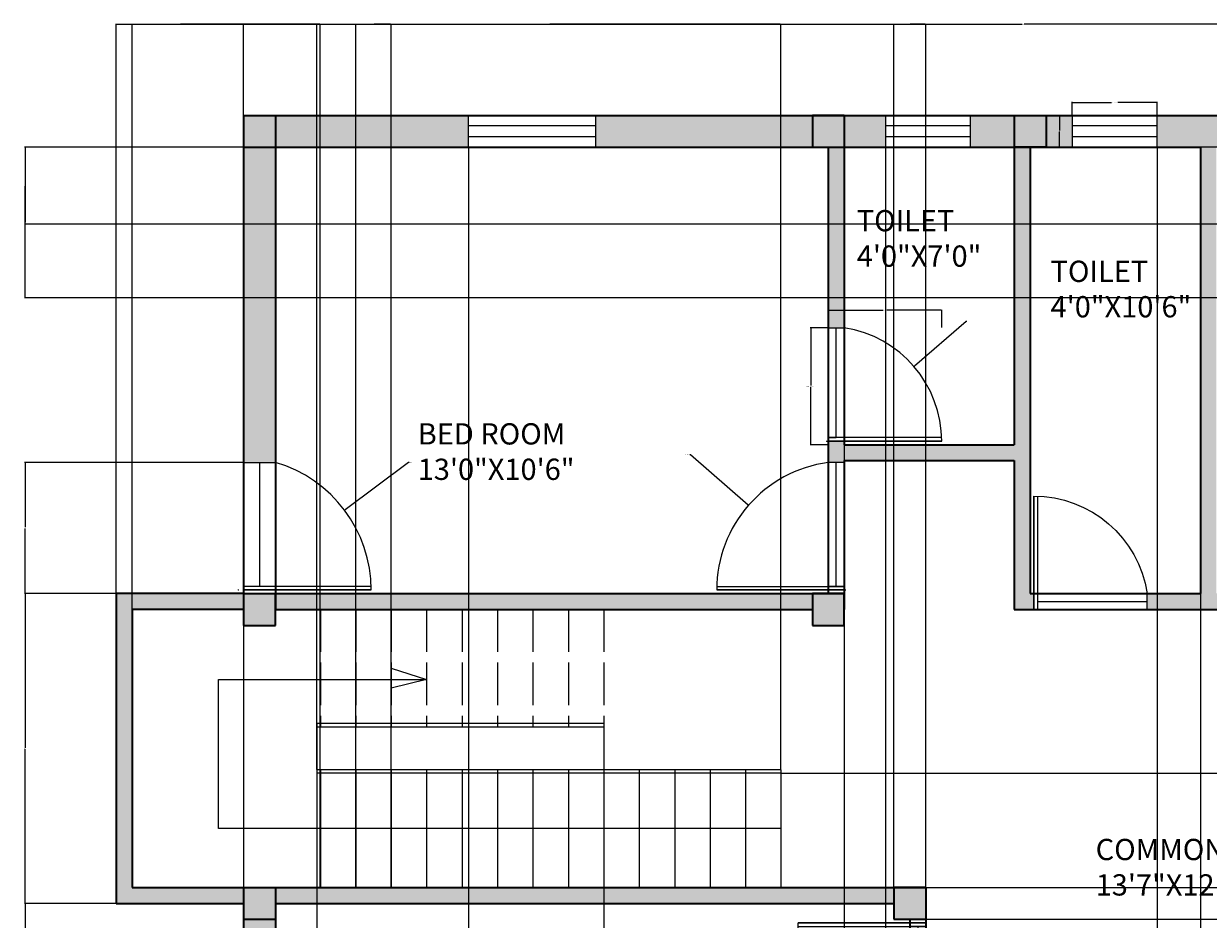
# Model space of a CAD drawing. Units: inches. Extents: x 6217 to 6782, y 16564 to 16973.
# Tile 2 of 3: x 6217 to 6552, y 16720 to 16973. Entities that reach past the tile are written whole.
import ezdxf

# ---------------------------------------------------------------- set-up
doc = ezdxf.new("R2010")
doc.units = ezdxf.units.IN
doc.header["$MEASUREMENT"] = 0
doc.linetypes.add('ACAD_ISO02W100', pattern=[15, 12, -3])
for name, color, linetype, lineweight in [('A-ANNO-DIMS', 2, 'Continuous', 18), ('A-ANNO-SYMB', 7, 'Continuous', 18), ('A-AREA-IDEN', 7, 'Continuous', 18), ('A-COLS', 7, 'Continuous', 35), ('A-DOOR', 3, 'Continuous', 18), ('A-FLOR-STRS', 7, 'Continuous', 25), ('A-FLOR-STRS-OVHD', 7, 'ACAD_ISO02W100', 18), ('A-GLAZ', 4, 'Continuous', 18), ('A-WALL', 7, 'Continuous', 35)]:
    doc.layers.add(name, color=color, linetype=linetype, lineweight=lineweight)
doc.layers.add('A-COLS-PATT', color=252, linetype='Continuous', lineweight=13, true_color=0x939598)
doc.layers.add('A-WALL-PATT', color=146, linetype='Continuous', lineweight=13, true_color=0x105689)
doc.styles.get("Standard").update_dxf_attribs({"font": 'arial.ttf'})
doc.dimstyles.get("Standard").update_dxf_attribs({"dimtxt": 0.18, "dimasz": 0.18, "dimexe": 0.18, "dimexo": 0.0625, "dimgap": 0.09, "dimtad": 0, "dimtih": 1, "dimtoh": 1, "dimdec": 4, "dimzin": 0, "dimdsep": 46, "dimtxsty": 'Standard', "dimcen": 0.09, "dimadec": 0, "dimazin": 0, "dimtfac": 1, "dimtdec": 4, "dimtofl": 0, "dimtmove": 0, "dimatfit": 3, "dimfxl": 1, "dimtolj": 1, "dimtzin": 0, "dimarcsym": 0})

# ---------------------------------------------------------------- blocks, each defined once
blk = doc.blocks.new('WIN-36')
for p, q in [((0, 9), (0, 0)), ((36, 9), (0, 9)), ((36, 0), (36, 9)), ((36, 6), (0, 6)), ((0, 3), (36, 3)), ((0, 0), (36, 0))]:
    blk.add_line(p, q)
blk = doc.blocks.new('VENT-24')
for p, q in [((0, 9), (0, 0)), ((24, 9), (0, 9)), ((24, 0), (24, 9)), ((24, 6), (0, 6)), ((0, 3), (24, 3)), ((0, 0), (24, 0))]:
    blk.add_line(p, q)
blk = doc.blocks.new('DOOR-SINGLE-36-A')
for p, q in [((0, 36), (-4.5, 36)), ((-2.25, 1), (-2.25, 36)), ((0, 0), (0, 36)), ((-36, 1), (0, 1)), ((0, 0), (-36, 0)), ((-36, 0), (0, 0)), ((0, 1), (-4.5, 1)), ((-4.5, 1), (-2.25, 1)), ((0, -1), (0, 0))]:
    blk.add_line(p, q)
blk.add_arc((0.32, 0), 36.32, 97.6281, 180)
blk = doc.blocks.new('DOOR-SINGLE-32')
for p, q in [((0, 0), (0, 32)), ((0, 32), (4.5, 32)), ((2.25, 1), (2.25, 32)), ((32, 1), (0, 1)), ((4.5, 1), (0, 1)), ((0, -1), (0, 0)), ((0, 0), (32, 0)), ((32, 0), (0, 0))]:
    blk.add_line(p, q)
blk.add_arc((-0.37, 0), 32.37, 0, 81.3499)
blk = doc.blocks.new('*D8')
at = {"layer": 'A-ANNO-DIMS', "color": 0, "lineweight": -2, "transparency": 16777216}
for p, q in [((6513.38, 16947.07), (6513.38, 16950.78)), ((6513.56, 16950.6), (6524.48, 16950.6)), ((6537.2, 16950.6), (6526.28, 16950.6)), ((6537.38, 16947.07), (6537.38, 16950.78))]:
    blk.add_line(p, q, dxfattribs=at)
at = {"layer": 'A-ANNO-DIMS', "color": 0, "transparency": 16777216}
for points in [[(6513.56, 16950.63), (6513.56, 16950.57), (6513.38, 16950.6)], [(6537.2, 16950.63), (6537.2, 16950.57), (6537.38, 16950.6)]]:
    blk.add_solid(points, dxfattribs=at)
at = {"layer": 'Defpoints', "color": 0, "transparency": 16777216}
for p in [(6513.38, 16950.6), (6513.38, 16947), (6537.38, 16947)]:
    blk.add_point(p, dxfattribs=at)
at = {"layer": 'A-ANNO-DIMS', "color": 0, "transparency": 16777216, "insert": (6525.38, 16950.6), "char_height": 0.18, "attachment_point": 5}
blk.add_mtext('\\A1;VENT 24 TYP.', dxfattribs=at)
blk = doc.blocks.new('*D9')
at = {"layer": 'A-ANNO-DIMS', "color": 0, "lineweight": -2, "transparency": 16777216}
for p, q in [((6513.32, 16947), (6509.6, 16947)), ((6509.78, 16946.82), (6509.78, 16942.69)), ((6509.78, 16938.18), (6509.78, 16942.32)), ((6513.32, 16938), (6509.6, 16938))]:
    blk.add_line(p, q, dxfattribs=at)
at = {"layer": 'A-ANNO-DIMS', "color": 0, "transparency": 16777216}
for points in [[(6509.75, 16946.82), (6509.81, 16946.82), (6509.78, 16947)], [(6509.75, 16938.18), (6509.81, 16938.18), (6509.78, 16938)]]:
    blk.add_solid(points, dxfattribs=at)
at = {"layer": 'Defpoints', "color": 0, "transparency": 16777216}
for p in [(6513.38, 16947), (6509.78, 16938), (6513.38, 16938)]:
    blk.add_point(p, dxfattribs=at)
at = {"layer": 'A-ANNO-DIMS', "color": 0, "transparency": 16777216, "insert": (6509.78, 16942.5), "char_height": 0.18, "attachment_point": 5}
blk.add_mtext('\\A1;9 TYP.', dxfattribs=at)
blk = doc.blocks.new('*D14')
at = {"layer": 'A-ANNO-DIMS', "color": 0, "lineweight": -2, "transparency": 16777216}
for p, q in [((6444.47, 16887), (6439.4, 16887)), ((6439.58, 16886.82), (6439.58, 16870.69)), ((6439.58, 16854.18), (6439.58, 16870.32)), ((6444.47, 16854), (6439.4, 16854))]:
    blk.add_line(p, q, dxfattribs=at)
at = {"layer": 'A-ANNO-DIMS', "color": 0, "transparency": 16777216}
for points in [[(6439.55, 16886.82), (6439.61, 16886.82), (6439.58, 16887)], [(6439.55, 16854.18), (6439.61, 16854.18), (6439.58, 16854)]]:
    blk.add_solid(points, dxfattribs=at)
at = {"layer": 'Defpoints', "color": 0, "transparency": 16777216}
for p in [(6439.58, 16887), (6444.53, 16887), (6444.53, 16854)]:
    blk.add_point(p, dxfattribs=at)
at = {"layer": 'A-ANNO-DIMS', "color": 0, "transparency": 16777216, "insert": (6439.58, 16870.5), "char_height": 0.18, "attachment_point": 5}
blk.add_mtext('\\A1;BATH DOOR 33 TYP.', dxfattribs=at)
blk = doc.blocks.new('*D15')
at = {"layer": 'A-ANNO-DIMS', "color": 0, "lineweight": -2, "transparency": 16777216}
for p, q in [((6444.53, 16887.07), (6444.53, 16892.13)), ((6444.71, 16891.95), (6460, 16891.95)), ((6476.35, 16891.95), (6461.06, 16891.95)), ((6476.53, 16887.07), (6476.53, 16892.13))]:
    blk.add_line(p, q, dxfattribs=at)
at = {"layer": 'A-ANNO-DIMS', "color": 0, "transparency": 16777216}
for points in [[(6444.71, 16891.98), (6444.71, 16891.92), (6444.53, 16891.95)], [(6476.35, 16891.98), (6476.35, 16891.92), (6476.53, 16891.95)]]:
    blk.add_solid(points, dxfattribs=at)
at = {"layer": 'Defpoints', "color": 0, "transparency": 16777216}
for p in [(6476.53, 16891.95), (6444.53, 16887), (6476.53, 16887)]:
    blk.add_point(p, dxfattribs=at)
at = {"layer": 'A-ANNO-DIMS', "color": 0, "transparency": 16777216, "insert": (6460.53, 16891.95), "char_height": 0.18, "attachment_point": 5}
blk.add_mtext('\\A1;32 TYP.', dxfattribs=at)
blk = doc.blocks.new('*D16')
at = {"layer": 'A-ANNO-DIMS', "color": 0, "lineweight": -2, "transparency": 16777216}
for p, q in [((6243.53, 16812.07), (6243.53, 16972.89)), ((6243.71, 16972.71), (6499.24, 16972.71)), ((6755.35, 16972.71), (6499.82, 16972.71)), ((6755.53, 16947.07), (6755.53, 16972.89))]:
    blk.add_line(p, q, dxfattribs=at)
at = {"layer": 'A-ANNO-DIMS', "color": 0, "transparency": 16777216}
for points in [[(6243.71, 16972.74), (6243.71, 16972.68), (6243.53, 16972.71)], [(6755.35, 16972.74), (6755.35, 16972.68), (6755.53, 16972.71)]]:
    blk.add_solid(points, dxfattribs=at)
at = {"layer": 'Defpoints', "color": 0, "transparency": 16777216}
for p in [(6755.53, 16972.71), (6755.53, 16947), (6243.53, 16812)]:
    blk.add_point(p, dxfattribs=at)
at = {"layer": 'A-ANNO-DIMS', "color": 0, "transparency": 16777216, "insert": (6499.53, 16972.71), "char_height": 0.18, "attachment_point": 5}
blk.add_mtext('\\A1;512', dxfattribs=at)
blk = doc.blocks.new('*D18')
at = {"layer": 'A-ANNO-DIMS', "color": 0, "lineweight": -2, "transparency": 16777216}
for p, q in [((6243.53, 16812.07), (6243.53, 16972.89)), ((6243.71, 16972.71), (6261.31, 16972.71)), ((6279.35, 16972.71), (6261.75, 16972.71)), ((6279.53, 16812.07), (6279.53, 16972.89))]:
    blk.add_line(p, q, dxfattribs=at)
at = {"layer": 'A-ANNO-DIMS', "color": 0, "transparency": 16777216}
for points in [[(6243.71, 16972.74), (6243.71, 16972.68), (6243.53, 16972.71)], [(6279.35, 16972.74), (6279.35, 16972.68), (6279.53, 16972.71)]]:
    blk.add_solid(points, dxfattribs=at)
at = {"layer": 'Defpoints', "color": 0, "transparency": 16777216}
for p in [(6279.53, 16972.71), (6243.53, 16812), (6279.53, 16812)]:
    blk.add_point(p, dxfattribs=at)
at = {"layer": 'A-ANNO-DIMS', "color": 0, "transparency": 16777216, "insert": (6261.53, 16972.71), "char_height": 0.18, "attachment_point": 5}
blk.add_mtext('\\A1;36', dxfattribs=at)
blk = doc.blocks.new('*D19')
at = {"layer": 'A-ANNO-DIMS', "color": 0, "lineweight": -2, "transparency": 16777216}
for p, q in [((6243.47, 16812), (6217.65, 16812)), ((6217.83, 16811.82), (6217.83, 16768.44)), ((6217.83, 16724.68), (6217.83, 16768.07)), ((6243.47, 16724.5), (6217.65, 16724.5))]:
    blk.add_line(p, q, dxfattribs=at)
at = {"layer": 'A-ANNO-DIMS', "color": 0, "transparency": 16777216}
for points in [[(6217.8, 16811.82), (6217.86, 16811.82), (6217.83, 16812)], [(6217.8, 16724.68), (6217.86, 16724.68), (6217.83, 16724.5)]]:
    blk.add_solid(points, dxfattribs=at)
at = {"layer": 'Defpoints', "color": 0, "transparency": 16777216}
for p in [(6217.83, 16812), (6243.53, 16812), (6243.53, 16724.5)]:
    blk.add_point(p, dxfattribs=at)
at = {"layer": 'A-ANNO-DIMS', "color": 0, "transparency": 16777216, "insert": (6217.83, 16768.25), "char_height": 0.18, "attachment_point": 5}
blk.add_mtext('\\A1;87.5', dxfattribs=at)
blk = doc.blocks.new('*D20')
at = {"layer": 'A-ANNO-DIMS', "color": 0, "lineweight": -2, "transparency": 16777216}
for p, q in [((6279.47, 16724.5), (6217.65, 16724.5)), ((6217.83, 16724.32), (6217.83, 16657.19)), ((6217.83, 16589.68), (6217.83, 16656.82)), ((6279.47, 16589.5), (6217.65, 16589.5))]:
    blk.add_line(p, q, dxfattribs=at)
at = {"layer": 'A-ANNO-DIMS', "color": 0, "transparency": 16777216}
for points in [[(6217.8, 16724.32), (6217.86, 16724.32), (6217.83, 16724.5)], [(6217.8, 16589.68), (6217.86, 16589.68), (6217.83, 16589.5)]]:
    blk.add_solid(points, dxfattribs=at)
at = {"layer": 'Defpoints', "color": 0, "transparency": 16777216}
for p in [(6217.83, 16724.5), (6279.53, 16724.5), (6279.53, 16589.5)]:
    blk.add_point(p, dxfattribs=at)
at = {"layer": 'A-ANNO-DIMS', "color": 0, "transparency": 16777216, "insert": (6217.83, 16657), "char_height": 0.18, "attachment_point": 5}
blk.add_mtext('\\A1;135', dxfattribs=at)
blk = doc.blocks.new('*D21')
at = {"layer": 'A-ANNO-DIMS', "color": 0, "lineweight": -2, "transparency": 16777216}
for p, q in [((6279.53, 16937.94), (6279.53, 16563.62)), ((6342.94, 16937.94), (6342.94, 16563.62)), ((6279.71, 16563.8), (6310.86, 16563.8)), ((6342.76, 16563.8), (6311.61, 16563.8))]:
    blk.add_line(p, q, dxfattribs=at)
at = {"layer": 'A-ANNO-DIMS', "color": 0, "transparency": 16777216}
for points in [[(6279.71, 16563.83), (6279.71, 16563.77), (6279.53, 16563.8)], [(6342.76, 16563.83), (6342.76, 16563.77), (6342.94, 16563.8)]]:
    blk.add_solid(points, dxfattribs=at)
at = {"layer": 'Defpoints', "color": 0, "transparency": 16777216}
for p in [(6279.53, 16938), (6342.94, 16938), (6342.94, 16563.8)]:
    blk.add_point(p, dxfattribs=at)
at = {"layer": 'A-ANNO-DIMS', "color": 0, "transparency": 16777216, "insert": (6311.23, 16563.8), "char_height": 0.18, "attachment_point": 5}
blk.add_mtext('\\A1;63.41', dxfattribs=at)
blk = doc.blocks.new('*D22')
at = {"layer": 'A-ANNO-DIMS', "color": 0, "lineweight": -2, "transparency": 16777216}
for p, q in [((6449.03, 16937.94), (6449.03, 16563.62)), ((6460.63, 16937.94), (6460.63, 16563.62)), ((6449.21, 16563.8), (6454.51, 16563.8)), ((6460.45, 16563.8), (6455.14, 16563.8))]:
    blk.add_line(p, q, dxfattribs=at)
at = {"layer": 'A-ANNO-DIMS', "color": 0, "transparency": 16777216}
for points in [[(6449.21, 16563.83), (6449.21, 16563.77), (6449.03, 16563.8)], [(6460.45, 16563.83), (6460.45, 16563.77), (6460.63, 16563.8)]]:
    blk.add_solid(points, dxfattribs=at)
at = {"layer": 'Defpoints', "color": 0, "transparency": 16777216}
for p in [(6449.03, 16938), (6460.63, 16938), (6460.63, 16563.8)]:
    blk.add_point(p, dxfattribs=at)
at = {"layer": 'A-ANNO-DIMS', "color": 0, "transparency": 16777216, "insert": (6454.83, 16563.8), "char_height": 0.18, "attachment_point": 5}
blk.add_mtext('\\A1;11.6', dxfattribs=at)
blk = doc.blocks.new('*D23')
at = {"layer": 'A-ANNO-DIMS', "color": 0, "lineweight": -2, "transparency": 16777216}
for p, q in [((6537.38, 16937.94), (6537.38, 16563.62)), ((6549.53, 16937.94), (6549.53, 16563.62)), ((6537.56, 16563.8), (6543, 16563.8)), ((6549.35, 16563.8), (6543.91, 16563.8))]:
    blk.add_line(p, q, dxfattribs=at)
at = {"layer": 'A-ANNO-DIMS', "color": 0, "transparency": 16777216}
for points in [[(6537.56, 16563.83), (6537.56, 16563.77), (6537.38, 16563.8)], [(6549.35, 16563.83), (6549.35, 16563.77), (6549.53, 16563.8)]]:
    blk.add_solid(points, dxfattribs=at)
at = {"layer": 'Defpoints', "color": 0, "transparency": 16777216}
for p in [(6537.38, 16938), (6549.53, 16938), (6549.53, 16563.8)]:
    blk.add_point(p, dxfattribs=at)
at = {"layer": 'A-ANNO-DIMS', "color": 0, "transparency": 16777216, "insert": (6543.45, 16563.8), "char_height": 0.18, "attachment_point": 5}
blk.add_mtext('\\A1;12.147', dxfattribs=at)
blk = doc.blocks.new('*D26')
at = {"layer": 'A-ANNO-DIMS', "color": 0, "lineweight": -2, "transparency": 16777216}
for p, q in [((6755.47, 16938), (6217.65, 16938)), ((6217.83, 16937.82), (6217.83, 16916.95)), ((6217.83, 16895.7), (6217.83, 16916.58)), ((6746.47, 16895.52), (6217.65, 16895.52))]:
    blk.add_line(p, q, dxfattribs=at)
at = {"layer": 'A-ANNO-DIMS', "color": 0, "transparency": 16777216}
for points in [[(6217.8, 16937.82), (6217.86, 16937.82), (6217.83, 16938)], [(6217.8, 16895.7), (6217.86, 16895.7), (6217.83, 16895.52)]]:
    blk.add_solid(points, dxfattribs=at)
at = {"layer": 'Defpoints', "color": 0, "transparency": 16777216}
for p in [(6755.53, 16938), (6217.83, 16895.52), (6746.53, 16895.52)]:
    blk.add_point(p, dxfattribs=at)
at = {"layer": 'A-ANNO-DIMS', "color": 0, "transparency": 16777216, "insert": (6217.83, 16916.76), "char_height": 0.18, "attachment_point": 5}
blk.add_mtext('\\A1;42.48', dxfattribs=at)
blk = doc.blocks.new('*D33')
at = {"layer": 'A-ANNO-DIMS', "color": 0, "lineweight": -2, "transparency": 16777216}
for p, q in [((6300.17, 16762.32), (6300.17, 16972.89)), ((6300.35, 16972.71), (6365.41, 16972.71)), ((6430.99, 16972.71), (6365.94, 16972.71)), ((6431.17, 16762.32), (6431.17, 16972.89))]:
    blk.add_line(p, q, dxfattribs=at)
at = {"layer": 'A-ANNO-DIMS', "color": 0, "transparency": 16777216}
for points in [[(6300.35, 16972.74), (6300.35, 16972.68), (6300.17, 16972.71)], [(6430.99, 16972.74), (6430.99, 16972.68), (6431.17, 16972.71)]]:
    blk.add_solid(points, dxfattribs=at)
at = {"layer": 'Defpoints', "color": 0, "transparency": 16777216}
for p in [(6431.17, 16972.71), (6300.17, 16762.25), (6431.17, 16762.25)]:
    blk.add_point(p, dxfattribs=at)
at = {"layer": 'A-ANNO-DIMS', "color": 0, "transparency": 16777216, "insert": (6365.67, 16972.71), "char_height": 0.18, "attachment_point": 5}
blk.add_mtext('\\A1;131', dxfattribs=at)
blk = doc.blocks.new('*D34')
at = {"layer": 'A-ANNO-DIMS', "color": 0, "lineweight": -2, "transparency": 16777216}
for p, q in [((6311.17, 16729.07), (6311.17, 16972.89)), ((6311.35, 16972.71), (6315.96, 16972.71)), ((6320.99, 16972.71), (6316.38, 16972.71)), ((6321.17, 16729.07), (6321.17, 16972.89))]:
    blk.add_line(p, q, dxfattribs=at)
at = {"layer": 'A-ANNO-DIMS', "color": 0, "transparency": 16777216}
for points in [[(6311.35, 16972.74), (6311.35, 16972.68), (6311.17, 16972.71)], [(6320.99, 16972.74), (6320.99, 16972.68), (6321.17, 16972.71)]]:
    blk.add_solid(points, dxfattribs=at)
at = {"layer": 'Defpoints', "color": 0, "transparency": 16777216}
for p in [(6321.17, 16972.71), (6311.17, 16729), (6321.17, 16729)]:
    blk.add_point(p, dxfattribs=at)
at = {"layer": 'A-ANNO-DIMS', "color": 0, "transparency": 16777216, "insert": (6316.17, 16972.71), "char_height": 0.18, "attachment_point": 5}
blk.add_mtext('\\A1;10', dxfattribs=at)
blk = doc.blocks.new('*D35')
at = {"layer": 'A-ANNO-DIMS', "color": 0, "lineweight": -2, "transparency": 16777216}
for p, q in [((6431.24, 16761.25), (6781.41, 16761.25)), ((6781.23, 16761.07), (6781.23, 16745.31)), ((6781.23, 16729.18), (6781.23, 16744.95)), ((6431.24, 16729), (6781.41, 16729))]:
    blk.add_line(p, q, dxfattribs=at)
at = {"layer": 'A-ANNO-DIMS', "color": 0, "transparency": 16777216}
for points in [[(6781.2, 16761.07), (6781.26, 16761.07), (6781.23, 16761.25)], [(6781.2, 16729.18), (6781.26, 16729.18), (6781.23, 16729)]]:
    blk.add_solid(points, dxfattribs=at)
at = {"layer": 'Defpoints', "color": 0, "transparency": 16777216}
for p in [(6431.17, 16761.25), (6781.23, 16761.25), (6431.17, 16729)]:
    blk.add_point(p, dxfattribs=at)
at = {"layer": 'A-ANNO-DIMS', "color": 0, "transparency": 16777216, "insert": (6781.23, 16745.13), "char_height": 0.18, "attachment_point": 5}
blk.add_mtext('\\A1;32.25', dxfattribs=at)
blk = doc.blocks.new('*D36')
at = {"layer": 'A-ANNO-DIMS', "color": 0, "lineweight": -2, "transparency": 16777216}
for p, q in [((6248.03, 16729.07), (6248.03, 16972.89)), ((6248.21, 16972.71), (6274.21, 16972.71)), ((6300.99, 16972.71), (6275, 16972.71)), ((6301.17, 16729.07), (6301.17, 16972.89))]:
    blk.add_line(p, q, dxfattribs=at)
at = {"layer": 'A-ANNO-DIMS', "color": 0, "transparency": 16777216}
for points in [[(6248.21, 16972.74), (6248.21, 16972.68), (6248.03, 16972.71)], [(6300.99, 16972.74), (6300.99, 16972.68), (6301.17, 16972.71)]]:
    blk.add_solid(points, dxfattribs=at)
at = {"layer": 'Defpoints', "color": 0, "transparency": 16777216}
for p in [(6301.17, 16972.71), (6248.03, 16729), (6301.17, 16729)]:
    blk.add_point(p, dxfattribs=at)
at = {"layer": 'A-ANNO-DIMS', "color": 0, "transparency": 16777216, "insert": (6274.6, 16972.71), "char_height": 0.18, "attachment_point": 5}
blk.add_mtext('\\A1;53.15', dxfattribs=at)
blk = doc.blocks.new('*D37')
at = {"layer": 'A-ANNO-DIMS', "color": 0, "lineweight": -2, "transparency": 16777216}
for p, q in [((6300.17, 16774.19), (6300.17, 16563.62)), ((6381.17, 16774.19), (6381.17, 16563.62)), ((6300.35, 16563.8), (6340.47, 16563.8)), ((6380.99, 16563.8), (6340.88, 16563.8))]:
    blk.add_line(p, q, dxfattribs=at)
at = {"layer": 'A-ANNO-DIMS', "color": 0, "transparency": 16777216}
for points in [[(6300.35, 16563.83), (6300.35, 16563.77), (6300.17, 16563.8)], [(6380.99, 16563.83), (6380.99, 16563.77), (6381.17, 16563.8)]]:
    blk.add_solid(points, dxfattribs=at)
at = {"layer": 'Defpoints', "color": 0, "transparency": 16777216}
for p in [(6300.17, 16774.25), (6381.17, 16774.25), (6381.17, 16563.8)]:
    blk.add_point(p, dxfattribs=at)
at = {"layer": 'A-ANNO-DIMS', "color": 0, "transparency": 16777216, "insert": (6340.67, 16563.8), "char_height": 0.18, "attachment_point": 5}
blk.add_mtext('\\A1;81', dxfattribs=at)
blk = doc.blocks.new('*D39')
at = {"layer": 'A-ANNO-DIMS', "color": 0, "lineweight": -2, "transparency": 16777216}
for p, q in [((6633.97, 16938), (6217.65, 16938)), ((6217.83, 16937.82), (6217.83, 16927.33)), ((6217.83, 16916.48), (6217.83, 16926.97)), ((6633.97, 16916.3), (6217.65, 16916.3))]:
    blk.add_line(p, q, dxfattribs=at)
at = {"layer": 'A-ANNO-DIMS', "color": 0, "transparency": 16777216}
for points in [[(6217.8, 16937.82), (6217.86, 16937.82), (6217.83, 16938)], [(6217.8, 16916.48), (6217.86, 16916.48), (6217.83, 16916.3)]]:
    blk.add_solid(points, dxfattribs=at)
at = {"layer": 'Defpoints', "color": 0, "transparency": 16777216}
for p in [(6217.83, 16938), (6634.03, 16938), (6634.03, 16916.3)]:
    blk.add_point(p, dxfattribs=at)
at = {"layer": 'A-ANNO-DIMS', "color": 0, "transparency": 16777216, "insert": (6217.83, 16927.15), "char_height": 0.18, "attachment_point": 5}
blk.add_mtext('\\A1;21.706', dxfattribs=at)
blk = doc.blocks.new('*D41')
at = {"layer": 'A-ANNO-DIMS', "color": 0, "lineweight": -2, "transparency": 16777216}
for p, q in [((6463.03, 16729.07), (6463.03, 16972.89)), ((6463.21, 16972.71), (6467.38, 16972.71)), ((6471.85, 16972.71), (6467.68, 16972.71)), ((6472.03, 16729.07), (6472.03, 16972.89))]:
    blk.add_line(p, q, dxfattribs=at)
at = {"layer": 'A-ANNO-DIMS', "color": 0, "transparency": 16777216}
for points in [[(6463.21, 16972.74), (6463.21, 16972.68), (6463.03, 16972.71)], [(6471.85, 16972.74), (6471.85, 16972.68), (6472.03, 16972.71)]]:
    blk.add_solid(points, dxfattribs=at)
at = {"layer": 'Defpoints', "color": 0, "transparency": 16777216}
for p in [(6472.03, 16972.71), (6463.03, 16729), (6472.03, 16729)]:
    blk.add_point(p, dxfattribs=at)
at = {"layer": 'A-ANNO-DIMS', "color": 0, "transparency": 16777216, "insert": (6467.53, 16972.71), "char_height": 0.18, "attachment_point": 5}
blk.add_mtext('\\A1;9', dxfattribs=at)
blk = doc.blocks.new('*D42')
at = {"layer": 'A-ANNO-DIMS', "color": 0, "lineweight": -2, "transparency": 16777216}
for p, q in [((6472.09, 16729), (6781.41, 16729)), ((6781.23, 16728.82), (6781.23, 16724.69)), ((6781.23, 16720.18), (6781.23, 16724.32)), ((6472.09, 16720), (6781.41, 16720))]:
    blk.add_line(p, q, dxfattribs=at)
at = {"layer": 'A-ANNO-DIMS', "color": 0, "transparency": 16777216}
for points in [[(6781.2, 16728.82), (6781.26, 16728.82), (6781.23, 16729)], [(6781.2, 16720.18), (6781.26, 16720.18), (6781.23, 16720)]]:
    blk.add_solid(points, dxfattribs=at)
at = {"layer": 'Defpoints', "color": 0, "transparency": 16777216}
for p in [(6472.03, 16729), (6781.23, 16729), (6472.03, 16720)]:
    blk.add_point(p, dxfattribs=at)
at = {"layer": 'A-ANNO-DIMS', "color": 0, "transparency": 16777216, "insert": (6781.23, 16724.5), "char_height": 0.18, "attachment_point": 5}
blk.add_mtext('\\A1;9', dxfattribs=at)
blk = doc.blocks.new('*D43')
at = {"layer": 'A-ANNO-DIMS', "color": 0, "lineweight": -2, "transparency": 16777216}
for p, q in [((6279.47, 16849), (6217.65, 16849)), ((6217.83, 16848.82), (6217.83, 16830.69)), ((6217.83, 16812.18), (6217.83, 16830.32)), ((6279.47, 16812), (6217.65, 16812))]:
    blk.add_line(p, q, dxfattribs=at)
at = {"layer": 'A-ANNO-DIMS', "color": 0, "transparency": 16777216}
for points in [[(6217.8, 16848.82), (6217.86, 16848.82), (6217.83, 16849)], [(6217.8, 16812.18), (6217.86, 16812.18), (6217.83, 16812)]]:
    blk.add_solid(points, dxfattribs=at)
at = {"layer": 'Defpoints', "color": 0, "transparency": 16777216}
for p in [(6279.53, 16849), (6217.83, 16812), (6279.53, 16812)]:
    blk.add_point(p, dxfattribs=at)
at = {"layer": 'A-ANNO-DIMS', "color": 0, "transparency": 16777216, "insert": (6217.83, 16830.5), "char_height": 0.18, "attachment_point": 5}
blk.add_mtext('\\A1;37', dxfattribs=at)
blk = doc.blocks.new('*D44')
at = {"layer": 'A-ANNO-DIMS', "color": 0, "lineweight": -2, "transparency": 16777216}
for p, q in [((6326.03, 16849), (6308.17, 16835.61)), ((6326.21, 16849), (6326.03, 16849)), ((6277.94, 16813), (6278.12, 16813)), ((6278.03, 16812.91), (6278.03, 16813.09))]:
    blk.add_line(p, q, dxfattribs=at)
at = {"layer": 'A-ANNO-DIMS', "color": 0, "transparency": 16777216}
blk.add_solid([(6308.15, 16835.64), (6308.19, 16835.59), (6308.03, 16835.5)], dxfattribs=at)
at = {"layer": 'Defpoints', "color": 0, "transparency": 16777216}
for p in [(6308.03, 16835.5), (6278.03, 16813)]:
    blk.add_point(p, dxfattribs=at)
at = {"layer": 'A-ANNO-DIMS', "color": 0, "transparency": 16777216, "insert": (6326.62, 16849), "char_height": 0.18, "attachment_point": 5}
blk.add_mtext('\\A1;R37.5', dxfattribs=at)
blk = doc.blocks.new('*D45')
at = {"layer": 'A-ANNO-DIMS', "color": 0, "lineweight": -2, "transparency": 16777216}
for p, q in [((6405.43, 16851.27), (6405.61, 16851.27)), ((6405.61, 16851.27), (6421.88, 16837.04)), ((6449.26, 16813), (6449.44, 16813)), ((6449.35, 16812.91), (6449.35, 16813.09))]:
    blk.add_line(p, q, dxfattribs=at)
at = {"layer": 'A-ANNO-DIMS', "color": 0, "transparency": 16777216}
blk.add_solid([(6421.9, 16837.06), (6421.86, 16837.02), (6422.02, 16836.92)], dxfattribs=at)
at = {"layer": 'Defpoints', "color": 0, "transparency": 16777216}
for p in [(6422.02, 16836.92), (6449.35, 16813)]:
    blk.add_point(p, dxfattribs=at)
at = {"layer": 'A-ANNO-DIMS', "color": 0, "transparency": 16777216, "insert": (6404.76, 16851.27), "char_height": 0.18, "attachment_point": 5}
blk.add_mtext('\\A1;4X R36.32', dxfattribs=at)
blk = doc.blocks.new('*D46')
at = {"layer": 'A-ANNO-DIMS', "color": 0, "lineweight": -2, "transparency": 16777216}
for p, q in [((6483.44, 16888.76), (6468.85, 16876.22)), ((6483.62, 16888.76), (6483.44, 16888.76)), ((6444.07, 16855), (6444.25, 16855)), ((6444.16, 16854.91), (6444.16, 16855.09))]:
    blk.add_line(p, q, dxfattribs=at)
at = {"layer": 'A-ANNO-DIMS', "color": 0, "transparency": 16777216}
blk.add_solid([(6468.83, 16876.24), (6468.86, 16876.19), (6468.71, 16876.1)], dxfattribs=at)
at = {"layer": 'Defpoints', "color": 0, "transparency": 16777216}
for p in [(6468.71, 16876.1), (6444.16, 16855)]:
    blk.add_point(p, dxfattribs=at)
at = {"layer": 'A-ANNO-DIMS', "color": 0, "transparency": 16777216, "insert": (6484.1, 16888.76), "char_height": 0.18, "attachment_point": 5}
blk.add_mtext('\\A1;R32.37', dxfattribs=at)

msp = doc.modelspace()

# ---------------------------------------------------------------- hatches: boundary and pattern name
at = {"layer": 'A-COLS-PATT'}
h = msp.add_hatch(color=256, dxfattribs=at)
h.dxf.hatch_style = 1
h.paths.add_polyline_path([(6288.5285, 16947.0033), (6279.5285, 16947.0033), (6279.5285, 16938.0033), (6288.5285, 16938.0033)])
h.paths.add_polyline_path([(6449.0285, 16947.0033), (6440.0285, 16947.0033), (6440.0285, 16938.0033), (6449.0285, 16938.0033)])
h.paths.add_polyline_path([(6506.0285, 16947.0033), (6497.0285, 16947.0033), (6497.0285, 16938.0033), (6506.0285, 16938.0033)])
h.paths.add_polyline_path([(6643.0285, 16947.0033), (6634.0285, 16947.0033), (6634.0285, 16938.0033), (6643.0285, 16938.0033)])
h.paths.add_polyline_path([(6755.5285, 16947.0033), (6746.5285, 16947.0033), (6746.5285, 16938.0033), (6755.5285, 16938.0033)])
h.paths.add_polyline_path([(6755.5285, 16770.0033), (6746.5285, 16770.0033), (6746.5285, 16761.0033), (6755.5285, 16761.0033)])
h.paths.add_polyline_path([(6643.0285, 16770.0033), (6634.0285, 16770.0033), (6634.0285, 16761.0033), (6643.0285, 16761.0033)])
h.paths.add_polyline_path([(6755.5285, 16598.5033), (6746.5285, 16598.5033), (6746.5285, 16589.5033), (6755.5285, 16589.5033)])
h.paths.add_polyline_path([(6643.0285, 16598.5033), (6634.0285, 16598.5033), (6634.0285, 16589.5033), (6643.0285, 16589.5033)])
h.paths.add_polyline_path([(6517.0285, 16598.5033), (6508.0285, 16598.5033), (6508.0285, 16589.5033), (6517.0285, 16589.5033)])
h.paths.add_polyline_path([(6472.0285, 16598.5033), (6463.0285, 16598.5033), (6463.0285, 16589.5033), (6472.0285, 16589.5033)])
h.paths.add_polyline_path([(6472.0285, 16729.0033), (6463.0285, 16729.0033), (6463.0285, 16720.0033), (6472.0285, 16720.0033)])
h.paths.add_polyline_path([(6288.5285, 16598.5033), (6279.5285, 16598.5033), (6279.5285, 16589.5033), (6288.5285, 16589.5033)])
h.paths.add_polyline_path([(6288.5285, 16729.0033), (6279.5285, 16729.0033), (6279.5285, 16720.0033), (6288.5285, 16720.0033)])
h.paths.add_polyline_path([(6288.5285, 16812.0033), (6279.5285, 16812.0033), (6279.5285, 16803.0033), (6288.5285, 16803.0033)])
h.paths.add_polyline_path([(6449.0285, 16812.0033), (6440.0285, 16812.0033), (6440.0285, 16803.0033), (6449.0285, 16803.0033)])
at = {"layer": 'A-WALL-PATT'}
h = msp.add_hatch(color=256, dxfattribs=at)
h.dxf.hatch_style = 1
h.paths.add_polyline_path([(6497.0285, 16947.0033), (6484.6293, 16947.0033), (6484.6293, 16938.0033), (6497.0285, 16938.0033)])
h.paths.add_polyline_path([(6513.3814, 16947.0033), (6506.0285, 16947.0033), (6506.0285, 16938.0033), (6513.3814, 16938.0033)])
h.paths.add_polyline_path([(6572.828, 16947.0033), (6537.3814, 16947.0033), (6537.3814, 16938.0033), (6549.5285, 16938.0033), (6549.5285, 16812.0033), (6534.5285, 16812.0033), (6534.5285, 16807.5033), (6597.0285, 16807.5033), (6597.0285, 16812.0033), (6554.0285, 16812.0033), (6554.0285, 16938.0033), (6572.828, 16938.0033)])
h.paths.add_polyline_path([(6501.5285, 16938.0033), (6497.0285, 16938.0033), (6497.0285, 16854.0033), (6449.0285, 16854.0033), (6449.0285, 16855.0033), (6444.5285, 16855.0033), (6444.5285, 16854.0033), (6444.5285, 16849.0033), (6449.0285, 16849.0033), (6449.0285, 16849.5033), (6497.0285, 16849.5033), (6497.0285, 16807.5033), (6502.5285, 16807.5033), (6502.5285, 16812.0033), (6501.5285, 16812.0033)])
h.paths.add_polyline_path([(6634.0285, 16947.0033), (6608.828, 16947.0033), (6608.828, 16938.0033), (6634.0285, 16938.0033)])
h.paths.add_polyline_path([(6664.4385, 16947.0033), (6643.0285, 16947.0033), (6643.0285, 16938.0033), (6664.4385, 16938.0033)])
h.paths.add_polyline_path([(6638.5285, 16938.0033), (6634.0285, 16938.0033), (6634.0285, 16812.0033), (6633.0285, 16812.0033), (6633.0285, 16807.5033), (6634.0285, 16807.5033), (6634.0285, 16807.0033), (6638.5285, 16807.0033)])
h.paths.add_polyline_path([(6746.5285, 16947.0033), (6700.4385, 16947.0033), (6700.4385, 16938.0033), (6746.5285, 16938.0033)])
h.paths.add_polyline_path([(6755.5285, 16938.0033), (6746.5285, 16938.0033), (6746.5285, 16895.525), (6755.5285, 16895.525)])
h.paths.add_polyline_path([(6755.5285, 16859.525), (6746.5285, 16859.525), (6746.5285, 16770.0033), (6755.5285, 16770.0033)])
h.paths.add_polyline_path([(6746.5285, 16770.0033), (6643.0285, 16770.0033), (6643.0285, 16765.5033), (6746.5285, 16765.5033)])
h.paths.add_polyline_path([(6755.5285, 16761.0033), (6746.5285, 16761.0033), (6746.5285, 16697.5292), (6755.5285, 16697.5292)])
h.paths.add_polyline_path([(6440.0285, 16812.0033), (6288.5285, 16812.0033), (6288.5285, 16807.5033), (6440.0285, 16807.5033)])
h.paths.add_polyline_path([(6288.5285, 16938.0033), (6279.5285, 16938.0033), (6279.5285, 16849.0033), (6288.5285, 16849.0033)])
h.paths.add_polyline_path([(6279.5285, 16729.0033), (6248.0285, 16729.0033), (6248.0285, 16807.5033), (6279.5285, 16807.5033), (6279.5285, 16812.0033), (6243.5285, 16812.0033), (6243.5285, 16724.5033), (6279.5285, 16724.5033)])
h.paths.add_polyline_path([(6463.0285, 16729.0033), (6288.5285, 16729.0033), (6288.5285, 16724.5033), (6463.0285, 16724.5033)])
h.paths.add_polyline_path([(6288.5285, 16720.0033), (6279.5285, 16720.0033), (6279.5285, 16679.7207), (6288.5285, 16679.7207)])
h.paths.add_polyline_path([(6288.5285, 16643.7207), (6279.5285, 16643.7207), (6279.5285, 16598.5033), (6288.5285, 16598.5033)])
h.paths.add_polyline_path([(6350.2697, 16598.5033), (6288.5285, 16598.5033), (6288.5285, 16589.5033), (6350.2697, 16589.5033)])
h.paths.add_polyline_path([(6463.0285, 16598.5033), (6386.2697, 16598.5033), (6386.2697, 16589.5033), (6463.0285, 16589.5033)])
h.paths.add_polyline_path([(6472.0285, 16683.0033), (6467.5285, 16683.0033), (6467.5285, 16598.5033), (6472.0285, 16598.5033)])
h.paths.add_polyline_path([(6532.5191, 16598.5033), (6517.0285, 16598.5033), (6517.0285, 16589.5033), (6532.5191, 16589.5033)])
h.paths.add_polyline_path([(6634.0285, 16598.5033), (6568.5191, 16598.5033), (6568.5191, 16589.5033), (6634.0285, 16589.5033)])
h.paths.add_polyline_path([(6661.0648, 16598.5033), (6643.0285, 16598.5033), (6643.0285, 16589.5033), (6661.0648, 16589.5033)])
h.paths.add_polyline_path([(6746.5285, 16598.5033), (6697.0648, 16598.5033), (6697.0648, 16589.5033), (6746.5285, 16589.5033)])
h.paths.add_polyline_path([(6755.5285, 16661.5292), (6746.5285, 16661.5292), (6746.5285, 16598.5033), (6755.5285, 16598.5033)])
h.paths.add_polyline_path([(6638.5285, 16724.0033), (6634.0285, 16724.0033), (6634.0285, 16598.5033), (6638.5285, 16598.5033)])
h = msp.add_hatch(color=256, dxfattribs=at)
h.dxf.hatch_style = 1
h.paths.add_polyline_path([(6342.9367, 16947.0033), (6288.5285, 16947.0033), (6288.5285, 16938.0033), (6342.9367, 16938.0033)])
h.paths.add_polyline_path([(6440.0285, 16947.0033), (6378.9367, 16947.0033), (6378.9367, 16938.0033), (6440.0285, 16938.0033)])
h.paths.add_polyline_path([(6460.6293, 16947.0033), (6449.0285, 16947.0033), (6449.0285, 16938.0033), (6460.6293, 16938.0033)])
h.paths.add_polyline_path([(6449.0285, 16938.0033), (6444.5285, 16938.0033), (6444.5285, 16887.0033), (6449.0285, 16887.0033)])

# ---------------------------------------------------------------- linework, layer by layer
at = {"layer": 'A-ANNO-SYMB'}
for p, q in [((6321.174, 16785.2433), (6321.174, 16790.8783)), ((6321.174, 16790.8783), (6331.174, 16787.6866)), ((6272.3838, 16745.6283), (6272.3838, 16787.6866)), ((6272.3838, 16787.6866), (6331.174, 16787.6866)), ((6331.174, 16787.6866), (6321.174, 16785.2433)), ((6431.174, 16745.6283), (6272.3838, 16745.6283))]:
    msp.add_line(p, q, dxfattribs=at)
at = {"layer": 'A-COLS'}
for p, q in [((6449.0285, 16947.0033), (6440.0285, 16947.0033)), ((6440.0285, 16947.0033), (6440.0285, 16938.0033)), ((6497.0285, 16947.0033), (6506.0285, 16947.0033)), ((6506.0285, 16947.0033), (6506.0285, 16938.0033)), ((6440.0285, 16938.0033), (6449.0285, 16938.0033)), ((6506.0285, 16938.0033), (6497.0285, 16938.0033)), ((6279.5285, 16812.0033), (6279.5285, 16803.0033)), ((6288.5285, 16803.0033), (6288.5285, 16812.0033)), ((6449.0285, 16812.0033), (6440.0285, 16812.0033)), ((6440.0285, 16812.0033), (6440.0285, 16803.0033)), ((6449.0285, 16803.0033), (6449.0285, 16812.0033)), ((6279.5285, 16803.0033), (6288.5285, 16803.0033)), ((6440.0285, 16803.0033), (6449.0285, 16803.0033)), ((6279.5285, 16729.0033), (6279.5285, 16720.0033)), ((6472.0285, 16729.0033), (6463.0285, 16729.0033)), ((6463.0285, 16729.0033), (6463.0285, 16720.0033)), ((6279.5285, 16720.0033), (6288.5285, 16720.0033)), ((6463.0285, 16720.0033), (6472.0285, 16720.0033))]:
    msp.add_line(p, q, dxfattribs=at)
at = {"layer": 'A-DOOR'}
for p, q in [((6444.5285, 16856.0033), (6446.7785, 16856.0033)), ((6279.5285, 16813.0033), (6279.5285, 16849.0033)), ((6279.5285, 16849.0033), (6288.5285, 16849.0033)), ((6284.0285, 16849.0033), (6284.0285, 16814.0033)), ((6315.5285, 16814.0033), (6279.5285, 16814.0033)), ((6279.5285, 16812.0033), (6279.5285, 16813.0033)), ((6279.5285, 16813.0033), (6315.5285, 16813.0033)), ((6315.5285, 16813.0033), (6279.5285, 16813.0033)), ((6503.5285, 16812.0033), (6503.5285, 16809.7533))]:
    msp.add_line(p, q, dxfattribs=at)
msp.add_arc((6278.0285, 16813.0033), 37.5, 0, 73.739795, dxfattribs=at)
at = {"layer": 'A-FLOR-STRS'}
for p, q in [((6381.174, 16775.2533), (6300.174, 16775.2533)), ((6300.174, 16775.2533), (6300.174, 16761.2533)), ((6381.174, 16774.2533), (6300.174, 16774.2533)), ((6431.174, 16762.2533), (6300.174, 16762.2533)), ((6431.174, 16761.2533), (6300.174, 16761.2533)), ((6301.174, 16762.2533), (6301.174, 16729.0033)), ((6311.174, 16762.2533), (6311.174, 16729.0033)), ((6321.174, 16762.2533), (6321.174, 16729.0033)), ((6331.174, 16762.2533), (6331.174, 16729.0033)), ((6341.174, 16762.2533), (6341.174, 16729.0033)), ((6351.174, 16762.2533), (6351.174, 16729.0033)), ((6361.174, 16762.2533), (6361.174, 16729.0033)), ((6371.174, 16762.2533), (6371.174, 16729.0033)), ((6381.174, 16762.2533), (6381.174, 16729.0033)), ((6391.174, 16762.2533), (6391.174, 16729.0033)), ((6401.174, 16762.2533), (6401.174, 16729.0033)), ((6411.174, 16762.2533), (6411.174, 16729.0033)), ((6421.174, 16762.2533), (6421.174, 16729.0033)), ((6431.174, 16762.2533), (6431.174, 16729.0033))]:
    msp.add_line(p, q, dxfattribs=at)
at = {"layer": 'A-FLOR-STRS-OVHD'}
for p, q in [((6301.174, 16807.5033), (6301.174, 16774.2533)), ((6311.174, 16807.5033), (6311.174, 16774.2533)), ((6321.174, 16807.5033), (6321.174, 16774.2533)), ((6331.174, 16807.5033), (6331.174, 16774.2533)), ((6341.174, 16807.5033), (6341.174, 16774.2533)), ((6351.174, 16807.5033), (6351.174, 16774.2533)), ((6361.174, 16807.5033), (6361.174, 16774.2533)), ((6371.174, 16807.5033), (6371.174, 16774.2533)), ((6381.174, 16807.5033), (6381.174, 16774.2533))]:
    msp.add_line(p, q, dxfattribs=at)
at = {"layer": 'A-WALL'}
for p, q in [((6279.5285, 16947.0033), (6755.5285, 16947.0033)), ((6279.5285, 16947.0033), (6279.5285, 16807.5033)), ((6288.5285, 16947.0033), (6288.5285, 16807.5033)), ((6449.0285, 16947.0033), (6449.0285, 16854.0033)), ((6497.0285, 16947.0033), (6497.0285, 16854.0033)), ((6279.5285, 16938.0033), (6549.5285, 16938.0033)), ((6444.5285, 16938.0033), (6444.5285, 16812.0033)), ((6501.5285, 16938.0033), (6501.5285, 16812.0033)), ((6549.5285, 16938.0033), (6549.5285, 16812.0033)), ((6449.0285, 16854.0033), (6497.0285, 16854.0033)), ((6449.0285, 16849.5033), (6497.0285, 16849.5033)), ((6449.0285, 16849.5033), (6449.0285, 16807.5033)), ((6497.0285, 16849.5033), (6497.0285, 16807.5033)), ((6279.5285, 16812.0033), (6243.5285, 16812.0033)), ((6243.5285, 16812.0033), (6243.5285, 16724.5033)), ((6279.5285, 16812.0033), (6449.0285, 16812.0033)), ((6279.5285, 16812.0033), (6449.0285, 16812.0033)), ((6501.5285, 16812.0033), (6549.5285, 16812.0033)), ((6248.0285, 16807.5033), (6248.0285, 16729.0033)), ((6279.5285, 16807.5033), (6248.0285, 16807.5033)), ((6288.5285, 16807.5033), (6440.0285, 16807.5033)), ((6288.5285, 16807.5033), (6440.0285, 16807.5033)), ((6497.0285, 16807.5033), (6634.0285, 16807.5033)), ((6248.0285, 16729.0033), (6279.5285, 16729.0033)), ((6279.5285, 16729.0033), (6472.0285, 16729.0033)), ((6279.5285, 16729.0033), (6279.5285, 16589.5033)), ((6288.5285, 16729.0033), (6288.5285, 16589.5033)), ((6472.0285, 16729.0033), (6472.0285, 16589.5033)), ((6243.5285, 16724.5033), (6279.5285, 16724.5033)), ((6288.5285, 16724.5033), (6463.0285, 16724.5033)), ((6467.5285, 16720.0033), (6467.5285, 16598.5033))]:
    msp.add_line(p, q, dxfattribs=at)

# ---------------------------------------------------------------- block references
at = {"layer": 'A-DOOR'}
for name, p in [('DOOR-SINGLE-32', (6444.5285, 16855.0033)), ('DOOR-SINGLE-36-A', (6449.0285, 16813.0033))]:
    msp.add_blockref(name, p, dxfattribs=at)
at = {"layer": 'A-DOOR', "extrusion": (0, 0, -1), "zscale": -1}
for name, p, rotation in [('DOOR-SINGLE-32', (-6502.5285, 16807.5033), 89.99999999999417), ('DOOR-SINGLE-36-A', (-6472.0285, 16719.0033), 180)]:
    msp.add_blockref(name, p, dxfattribs=dict(at, rotation=rotation))
at = {"layer": 'A-GLAZ'}
for name, p in [('WIN-36', (6342.9367, 16938.0033)), ('VENT-24', (6460.6293, 16938.0033))]:
    msp.add_blockref(name, p, dxfattribs=at)
at = {"layer": 'A-GLAZ', "rotation": 180}
msp.add_blockref('VENT-24', (6537.3814, 16947.0033), dxfattribs=at)

# ---------------------------------------------------------------- texts
at = {"layer": 'A-AREA-IDEN', "char_height": 6, "attachment_point": 1}
for s, width, insert in [('TOILET\\P4\'0"X7\'0"', 38.026586, (6452.5666, 16920.2617)), ('TOILET\\P4\'0"X10\'6"', 34.604214, (6507.2618, 16905.9632)), ('BED ROOM\\P13\'0"X10\'6"', 70.129186, (6328.6527, 16860.0685)), ('COMMON HALL\\P13\'7"X12\'6"', 74.34141, (6519.987, 16742.7201))]:
    msp.add_mtext_dynamic_manual_height_columns(s, width=width, gutter_width=1, heights=[0], dxfattribs=dict(at, insert=insert))

# ---------------------------------------------------------------- dimensions: what is measured, and where the dimension line sits
at = {"layer": 'A-ANNO-DIMS'}
for base, p1, p2, override, picture, middle in [((6755.5285, 16972.7058), (6243.5285, 16812.0033), (6755.5285, 16947.0033), {"dimdec": 0, "dimlfac": 1, "dimrnd": 0, "dimzin": 0, "dimdsep": 46, "dimlunit": 2}, '*D16', (6499.5285, 16972.7058)), ((6279.5285, 16972.7058), (6243.5285, 16812.0033), (6279.5285, 16812.0033), {"dimdec": 0, "dimlfac": 1, "dimrnd": 0, "dimzin": 0, "dimdsep": 46, "dimlunit": 2}, '*D18', (6261.5285, 16972.7058)), ((6301.174, 16972.7058), (6248.0285, 16729.0033), (6301.174, 16729.0033), {"dimdec": 2, "dimlfac": 1, "dimrnd": 0, "dimzin": 0, "dimdsep": 46, "dimlunit": 2}, '*D36', (6274.6012, 16972.7058)), ((6431.174, 16972.7058), (6300.174, 16762.2533), (6431.174, 16762.2533), {"dimdec": 0, "dimlfac": 1, "dimrnd": 0, "dimzin": 0, "dimdsep": 46, "dimlunit": 2}, '*D33', (6365.674, 16972.7058)), ((6321.174, 16972.7058), (6311.174, 16729.0033), (6321.174, 16729.0033), {"dimdec": 0, "dimlfac": 1, "dimrnd": 0, "dimzin": 0, "dimdsep": 46, "dimlunit": 2}, '*D34', (6316.174, 16972.7058)), ((6472.0285, 16972.7058), (6463.0285, 16729.0033), (6472.0285, 16729.0033), {"dimdec": 0, "dimlfac": 1, "dimrnd": 0, "dimzin": 0, "dimdsep": 46, "dimlunit": 2}, '*D41', (6467.5285, 16972.7058)), ((6342.9367, 16563.8008), (6279.5285, 16938.0033), (6342.9367, 16938.0033), {"dimdec": 2, "dimlfac": 1, "dimrnd": 0, "dimzin": 0, "dimdsep": 46, "dimlunit": 2}, '*D21', (6311.2326, 16563.8008)), ((6460.6293, 16563.8008), (6449.0285, 16938.0033), (6460.6293, 16938.0033), {"dimdec": 1, "dimlfac": 1, "dimrnd": 0, "dimzin": 0, "dimdsep": 46, "dimlunit": 2}, '*D22', (6454.8289, 16563.8008)), ((6549.5285, 16563.8008), (6537.3814, 16938.0033), (6549.5285, 16938.0033), {"dimdec": 3, "dimlfac": 1, "dimrnd": 0, "dimzin": 0, "dimdsep": 46, "dimlunit": 2}, '*D23', (6543.4549, 16563.8008)), ((6381.174, 16563.8008), (6300.174, 16774.2533), (6381.174, 16774.2533), {"dimdec": 0, "dimlfac": 1, "dimrnd": 0, "dimzin": 0, "dimdsep": 46, "dimlunit": 2}, '*D37', (6340.674, 16563.8008))]:
    dim = msp.add_linear_dim(base=base, p1=p1, p2=p2, dimstyle='Standard', override=override, dxfattribs=at)
    dim.commit()
    dim.dimension.update_dxf_attribs({"geometry": picture, "text_midpoint": middle})
for base, p1, p2, angle, text, picture, middle in [((6513.3814, 16950.6033), (6537.3814, 16947.0033), (6513.3814, 16947.0033), 180, 'VENT <> TYP.', '*D8', (6525.3814, 16950.6033)), ((6509.7814, 16938.0033), (6513.3814, 16947.0033), (6513.3814, 16938.0033), 270, '<> TYP.', '*D9', (6509.7814, 16942.5033)), ((6439.5785, 16887.0033), (6444.5285, 16854.0033), (6444.5285, 16887.0033), 90, 'BATH DOOR <> TYP.', '*D14', (6439.5785, 16870.5033))]:
    dim = msp.add_linear_dim(base=base, p1=p1, p2=p2, angle=angle, text=text, dimstyle='Standard', override={"dimdec": 0, "dimlfac": 1, "dimrnd": 0, "dimzin": 0, "dimdsep": 46, "dimlunit": 2}, dxfattribs=at)
    dim.commit()
    dim.dimension.update_dxf_attribs({"geometry": picture, "text_midpoint": middle})
for base, p1, p2, override, picture, middle in [((6217.826, 16938.00326), (6634.0285, 16916.29685), (6634.0285, 16938.00326), {"dimdec": 3, "dimlfac": 1, "dimrnd": 0, "dimzin": 0, "dimdsep": 46, "dimlunit": 2}, '*D39', (6217.826, 16927.15005)), ((6217.826, 16895.525), (6755.5285, 16938.0033), (6746.5285, 16895.525), {"dimdec": 2, "dimlfac": 1, "dimrnd": 0, "dimzin": 0, "dimdsep": 46, "dimlunit": 2}, '*D26', (6217.826, 16916.7641)), ((6217.826, 16812.0033), (6279.5285, 16849.0033), (6279.5285, 16812.0033), {"dimdec": 0, "dimlfac": 1, "dimrnd": 0, "dimzin": 0, "dimdsep": 46, "dimlunit": 2}, '*D43', (6217.826, 16830.5033)), ((6217.826, 16812.0033), (6243.5285, 16724.5033), (6243.5285, 16812.0033), {"dimdec": 1, "dimlfac": 1, "dimrnd": 0, "dimzin": 0, "dimdsep": 46, "dimlunit": 2}, '*D19', (6217.826, 16768.2533)), ((6781.231, 16761.2533), (6431.174, 16729.0033), (6431.174, 16761.2533), {"dimdec": 2, "dimlfac": 1, "dimrnd": 0, "dimzin": 0, "dimdsep": 46, "dimlunit": 2}, '*D35', (6781.231, 16745.1283)), ((6781.231, 16729.0033), (6472.0285, 16720.0033), (6472.0285, 16729.0033), {"dimdec": 0, "dimlfac": 1, "dimrnd": 0, "dimzin": 0, "dimdsep": 46, "dimlunit": 2}, '*D42', (6781.231, 16724.5033)), ((6217.826, 16724.5033), (6279.5285, 16589.5033), (6279.5285, 16724.5033), {"dimdec": 0, "dimlfac": 1, "dimrnd": 0, "dimzin": 0, "dimdsep": 46, "dimlunit": 2}, '*D20', (6217.826, 16657.0033))]:
    dim = msp.add_linear_dim(base=base, p1=p1, p2=p2, angle=90, dimstyle='Standard', override=override, dxfattribs=at)
    dim.commit()
    dim.dimension.update_dxf_attribs({"geometry": picture, "text_midpoint": middle})
dim = msp.add_linear_dim(base=(6476.5285, 16891.9533), p1=(6444.5285, 16887.0033), p2=(6476.5285, 16887.0033), text='<> TYP.', dimstyle='Standard', override={"dimdec": 0, "dimlfac": 1, "dimrnd": 0, "dimzin": 0, "dimdsep": 46, "dimlunit": 2}, dxfattribs=at)
dim.commit()
dim.dimension.update_dxf_attribs({"geometry": '*D15', "text_midpoint": (6460.5285, 16891.9533)})
for center, mpoint, override, picture, middle in [((6444.1603, 16855.0033), (6468.7089, 16876.0999), {"dimdec": 2, "dimlfac": 1, "dimrnd": 0, "dimzin": 0, "dimdsep": 46, "dimlunit": 2}, '*D46', (6484.0978, 16888.7579)), ((6278.0285, 16813.0033), (6308.0284, 16835.5033), {"dimdec": 1, "dimlfac": 1, "dimrnd": 0, "dimzin": 0, "dimdsep": 46, "dimlunit": 2}, '*D44', (6326.619, 16849.0034))]:
    dim = msp.add_radius_dim(center=center, mpoint=mpoint, dimstyle='Standard', override=override, dxfattribs=at)
    dim.commit()
    dim.dimension.update_dxf_attribs({"geometry": picture, "text_midpoint": middle, "dimtype": 164})
dim = msp.add_radius_dim(center=(6449.3499, 16813.0033), mpoint=(6422.0151, 16836.9209), text='4X <>', dimstyle='Standard', override={"dimdec": 2, "dimlfac": 1, "dimrnd": 0, "dimzin": 0, "dimdsep": 46, "dimlunit": 2}, dxfattribs=at)
dim.commit()
dim.dimension.update_dxf_attribs({"geometry": '*D45', "text_midpoint": (6404.7583, 16851.2715), "dimtype": 164})

doc.saveas('drawing.dxf')
